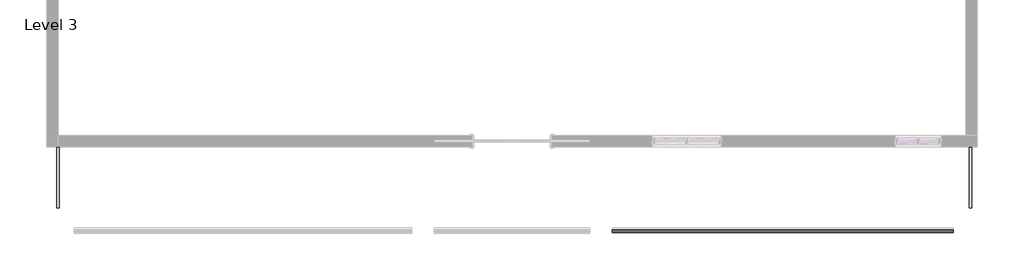
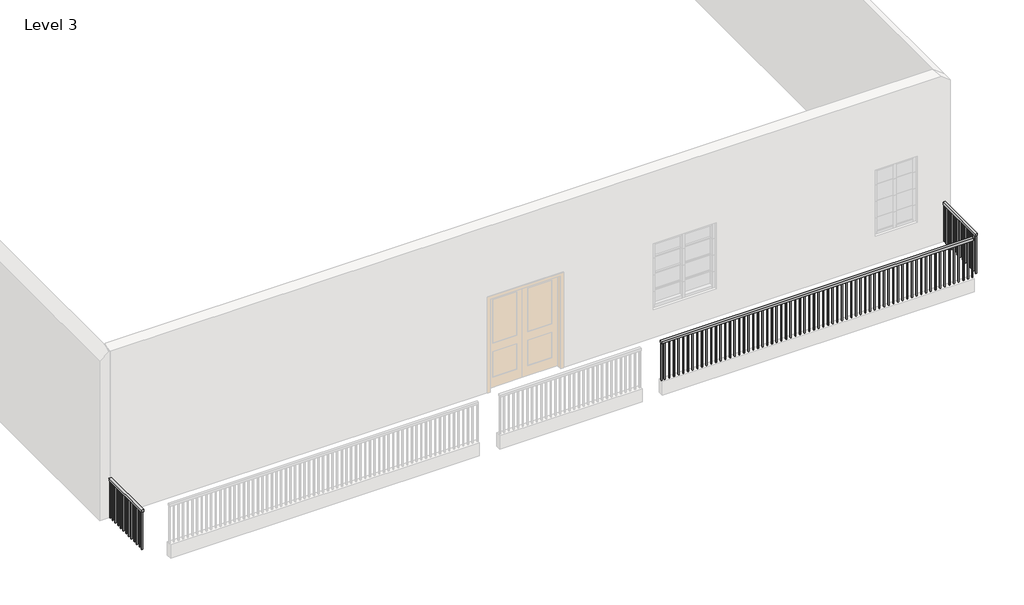
# One storey, part 3 of 3: 3 railings.
"""IFC4 building model written with IfcOpenShell, lengths in millimetres."""

from ifc_helpers import new_model, si_unit, frame, origin, place, context, project, spatial, polyline, outline, extrude, element, save

model = new_model("IFC4")

# Units and contexts
model_context = context("Model", 3, world=origin())
ifc_project = project(units=[si_unit("LENGTHUNIT", "METRE", prefix="MILLI")], contexts=[model_context])

# Site, building, storey
site = spatial("IfcSite", under=ifc_project)
building = spatial("IfcBuilding", under=site)
storey = spatial("IfcBuildingStorey", under=building, Name="Level 3", Elevation=3810.0)

# Railings
placement = place(None, origin())
element("IfcRailing", 1, ObjectType="Handrail - Rectangular", at=placement, inside=storey, context=model_context, shape_type="SweptSolid", body=[
    extrude(outline(polyline([(8263.5579341, -8749.7902135), (8263.5579341, -8800.5902135), (1481.7579341, -8800.5902135), (1481.7579341, -8749.7902135), (8263.5579341, -8749.7902135)])), frame((0.0, 0.0, 4978.4), z_axis=(0.0, 0.0, 1.0), x_axis=(1.0, 0.0, 0.0)), (0.0, 0.0, 1.0), 50.8),
    extrude(outline(polyline([(1567.4829341, -8765.6652135), (1567.4829341, -8784.7152135), (1548.4329341, -8784.7152135), (1548.4329341, -8765.6652135), (1567.4829341, -8765.6652135)])), frame((0.0, 0.0, 4114.8), z_axis=(0.0, 0.0, 1.0), x_axis=(1.0, 0.0, 0.0)), (0.0, 0.0, 1.0), 863.6),
    extrude(outline(polyline([(1669.0829341, -8765.6652135), (1669.0829341, -8784.7152135), (1650.0329341, -8784.7152135), (1650.0329341, -8765.6652135), (1669.0829341, -8765.6652135)])), frame((0.0, 0.0, 4114.8), z_axis=(0.0, 0.0, 1.0), x_axis=(1.0, 0.0, 0.0)), (0.0, 0.0, 1.0), 863.6),
    extrude(outline(polyline([(1770.6829341, -8765.6652135), (1770.6829341, -8784.7152135), (1751.6329341, -8784.7152135), (1751.6329341, -8765.6652135), (1770.6829341, -8765.6652135)])), frame((0.0, 0.0, 4114.8), z_axis=(0.0, 0.0, 1.0), x_axis=(1.0, 0.0, 0.0)), (0.0, 0.0, 1.0), 863.6),
    extrude(outline(polyline([(1872.2829341, -8765.6652135), (1872.2829341, -8784.7152135), (1853.2329341, -8784.7152135), (1853.2329341, -8765.6652135), (1872.2829341, -8765.6652135)])), frame((0.0, 0.0, 4114.8), z_axis=(0.0, 0.0, 1.0), x_axis=(1.0, 0.0, 0.0)), (0.0, 0.0, 1.0), 863.6),
    extrude(outline(polyline([(1973.8829341, -8765.6652135), (1973.8829341, -8784.7152135), (1954.8329341, -8784.7152135), (1954.8329341, -8765.6652135), (1973.8829341, -8765.6652135)])), frame((0.0, 0.0, 4114.8), z_axis=(0.0, 0.0, 1.0), x_axis=(1.0, 0.0, 0.0)), (0.0, 0.0, 1.0), 863.6),
    extrude(outline(polyline([(2075.4829341, -8765.6652135), (2075.4829341, -8784.7152135), (2056.4329341, -8784.7152135), (2056.4329341, -8765.6652135), (2075.4829341, -8765.6652135)])), frame((0.0, 0.0, 4114.8), z_axis=(0.0, 0.0, 1.0), x_axis=(1.0, 0.0, 0.0)), (0.0, 0.0, 1.0), 863.6),
    extrude(outline(polyline([(2177.0829341, -8765.6652135), (2177.0829341, -8784.7152135), (2158.0329341, -8784.7152135), (2158.0329341, -8765.6652135), (2177.0829341, -8765.6652135)])), frame((0.0, 0.0, 4114.8), z_axis=(0.0, 0.0, 1.0), x_axis=(1.0, 0.0, 0.0)), (0.0, 0.0, 1.0), 863.6),
    extrude(outline(polyline([(2278.6829341, -8765.6652135), (2278.6829341, -8784.7152135), (2259.6329341, -8784.7152135), (2259.6329341, -8765.6652135), (2278.6829341, -8765.6652135)])), frame((0.0, 0.0, 4114.8), z_axis=(0.0, 0.0, 1.0), x_axis=(1.0, 0.0, 0.0)), (0.0, 0.0, 1.0), 863.6),
    extrude(outline(polyline([(2380.2829341, -8765.6652135), (2380.2829341, -8784.7152135), (2361.2329341, -8784.7152135), (2361.2329341, -8765.6652135), (2380.2829341, -8765.6652135)])), frame((0.0, 0.0, 4114.8), z_axis=(0.0, 0.0, 1.0), x_axis=(1.0, 0.0, 0.0)), (0.0, 0.0, 1.0), 863.6),
    extrude(outline(polyline([(2481.8829341, -8765.6652135), (2481.8829341, -8784.7152135), (2462.8329341, -8784.7152135), (2462.8329341, -8765.6652135), (2481.8829341, -8765.6652135)])), frame((0.0, 0.0, 4114.8), z_axis=(0.0, 0.0, 1.0), x_axis=(1.0, 0.0, 0.0)), (0.0, 0.0, 1.0), 863.6),
    extrude(outline(polyline([(2583.4829341, -8765.6652135), (2583.4829341, -8784.7152135), (2564.4329341, -8784.7152135), (2564.4329341, -8765.6652135), (2583.4829341, -8765.6652135)])), frame((0.0, 0.0, 4114.8), z_axis=(0.0, 0.0, 1.0), x_axis=(1.0, 0.0, 0.0)), (0.0, 0.0, 1.0), 863.6),
    extrude(outline(polyline([(2685.0829341, -8765.6652135), (2685.0829341, -8784.7152135), (2666.0329341, -8784.7152135), (2666.0329341, -8765.6652135), (2685.0829341, -8765.6652135)])), frame((0.0, 0.0, 4114.8), z_axis=(0.0, 0.0, 1.0), x_axis=(1.0, 0.0, 0.0)), (0.0, 0.0, 1.0), 863.6),
    extrude(outline(polyline([(2786.6829341, -8765.6652135), (2786.6829341, -8784.7152135), (2767.6329341, -8784.7152135), (2767.6329341, -8765.6652135), (2786.6829341, -8765.6652135)])), frame((0.0, 0.0, 4114.8), z_axis=(0.0, 0.0, 1.0), x_axis=(1.0, 0.0, 0.0)), (0.0, 0.0, 1.0), 863.6),
    extrude(outline(polyline([(2888.2829341, -8765.6652135), (2888.2829341, -8784.7152135), (2869.2329341, -8784.7152135), (2869.2329341, -8765.6652135), (2888.2829341, -8765.6652135)])), frame((0.0, 0.0, 4114.8), z_axis=(0.0, 0.0, 1.0), x_axis=(1.0, 0.0, 0.0)), (0.0, 0.0, 1.0), 863.6),
    extrude(outline(polyline([(2989.8829341, -8765.6652135), (2989.8829341, -8784.7152135), (2970.8329341, -8784.7152135), (2970.8329341, -8765.6652135), (2989.8829341, -8765.6652135)])), frame((0.0, 0.0, 4114.8), z_axis=(0.0, 0.0, 1.0), x_axis=(1.0, 0.0, 0.0)), (0.0, 0.0, 1.0), 863.6),
    extrude(outline(polyline([(3091.4829341, -8765.6652135), (3091.4829341, -8784.7152135), (3072.4329341, -8784.7152135), (3072.4329341, -8765.6652135), (3091.4829341, -8765.6652135)])), frame((0.0, 0.0, 4114.8), z_axis=(0.0, 0.0, 1.0), x_axis=(1.0, 0.0, 0.0)), (0.0, 0.0, 1.0), 863.6),
    extrude(outline(polyline([(3193.0829341, -8765.6652135), (3193.0829341, -8784.7152135), (3174.0329341, -8784.7152135), (3174.0329341, -8765.6652135), (3193.0829341, -8765.6652135)])), frame((0.0, 0.0, 4114.8), z_axis=(0.0, 0.0, 1.0), x_axis=(1.0, 0.0, 0.0)), (0.0, 0.0, 1.0), 863.6),
    extrude(outline(polyline([(3294.6829341, -8765.6652135), (3294.6829341, -8784.7152135), (3275.6329341, -8784.7152135), (3275.6329341, -8765.6652135), (3294.6829341, -8765.6652135)])), frame((0.0, 0.0, 4114.8), z_axis=(0.0, 0.0, 1.0), x_axis=(1.0, 0.0, 0.0)), (0.0, 0.0, 1.0), 863.6),
    extrude(outline(polyline([(3396.2829341, -8765.6652135), (3396.2829341, -8784.7152135), (3377.2329341, -8784.7152135), (3377.2329341, -8765.6652135), (3396.2829341, -8765.6652135)])), frame((0.0, 0.0, 4114.8), z_axis=(0.0, 0.0, 1.0), x_axis=(1.0, 0.0, 0.0)), (0.0, 0.0, 1.0), 863.6),
    extrude(outline(polyline([(3497.8829341, -8765.6652135), (3497.8829341, -8784.7152135), (3478.8329341, -8784.7152135), (3478.8329341, -8765.6652135), (3497.8829341, -8765.6652135)])), frame((0.0, 0.0, 4114.8), z_axis=(0.0, 0.0, 1.0), x_axis=(1.0, 0.0, 0.0)), (0.0, 0.0, 1.0), 863.6),
    extrude(outline(polyline([(3599.4829341, -8765.6652135), (3599.4829341, -8784.7152135), (3580.4329341, -8784.7152135), (3580.4329341, -8765.6652135), (3599.4829341, -8765.6652135)])), frame((0.0, 0.0, 4114.8), z_axis=(0.0, 0.0, 1.0), x_axis=(1.0, 0.0, 0.0)), (0.0, 0.0, 1.0), 863.6),
    extrude(outline(polyline([(3701.0829341, -8765.6652135), (3701.0829341, -8784.7152135), (3682.0329341, -8784.7152135), (3682.0329341, -8765.6652135), (3701.0829341, -8765.6652135)])), frame((0.0, 0.0, 4114.8), z_axis=(0.0, 0.0, 1.0), x_axis=(1.0, 0.0, 0.0)), (0.0, 0.0, 1.0), 863.6),
    extrude(outline(polyline([(3802.6829341, -8765.6652135), (3802.6829341, -8784.7152135), (3783.6329341, -8784.7152135), (3783.6329341, -8765.6652135), (3802.6829341, -8765.6652135)])), frame((0.0, 0.0, 4114.8), z_axis=(0.0, 0.0, 1.0), x_axis=(1.0, 0.0, 0.0)), (0.0, 0.0, 1.0), 863.6),
    extrude(outline(polyline([(3904.2829341, -8765.6652135), (3904.2829341, -8784.7152135), (3885.2329341, -8784.7152135), (3885.2329341, -8765.6652135), (3904.2829341, -8765.6652135)])), frame((0.0, 0.0, 4114.8), z_axis=(0.0, 0.0, 1.0), x_axis=(1.0, 0.0, 0.0)), (0.0, 0.0, 1.0), 863.6),
    extrude(outline(polyline([(4005.8829341, -8765.6652135), (4005.8829341, -8784.7152135), (3986.8329341, -8784.7152135), (3986.8329341, -8765.6652135), (4005.8829341, -8765.6652135)])), frame((0.0, 0.0, 4114.8), z_axis=(0.0, 0.0, 1.0), x_axis=(1.0, 0.0, 0.0)), (0.0, 0.0, 1.0), 863.6),
    extrude(outline(polyline([(4107.4829341, -8765.6652135), (4107.4829341, -8784.7152135), (4088.4329341, -8784.7152135), (4088.4329341, -8765.6652135), (4107.4829341, -8765.6652135)])), frame((0.0, 0.0, 4114.8), z_axis=(0.0, 0.0, 1.0), x_axis=(1.0, 0.0, 0.0)), (0.0, 0.0, 1.0), 863.6),
    extrude(outline(polyline([(4209.0829341, -8765.6652135), (4209.0829341, -8784.7152135), (4190.0329341, -8784.7152135), (4190.0329341, -8765.6652135), (4209.0829341, -8765.6652135)])), frame((0.0, 0.0, 4114.8), z_axis=(0.0, 0.0, 1.0), x_axis=(1.0, 0.0, 0.0)), (0.0, 0.0, 1.0), 863.6),
    extrude(outline(polyline([(4310.6829341, -8765.6652135), (4310.6829341, -8784.7152135), (4291.6329341, -8784.7152135), (4291.6329341, -8765.6652135), (4310.6829341, -8765.6652135)])), frame((0.0, 0.0, 4114.8), z_axis=(0.0, 0.0, 1.0), x_axis=(1.0, 0.0, 0.0)), (0.0, 0.0, 1.0), 863.6),
    extrude(outline(polyline([(4412.2829341, -8765.6652135), (4412.2829341, -8784.7152135), (4393.2329341, -8784.7152135), (4393.2329341, -8765.6652135), (4412.2829341, -8765.6652135)])), frame((0.0, 0.0, 4114.8), z_axis=(0.0, 0.0, 1.0), x_axis=(1.0, 0.0, 0.0)), (0.0, 0.0, 1.0), 863.6),
    extrude(outline(polyline([(4513.8829341, -8765.6652135), (4513.8829341, -8784.7152135), (4494.8329341, -8784.7152135), (4494.8329341, -8765.6652135), (4513.8829341, -8765.6652135)])), frame((0.0, 0.0, 4114.8), z_axis=(0.0, 0.0, 1.0), x_axis=(1.0, 0.0, 0.0)), (0.0, 0.0, 1.0), 863.6),
    extrude(outline(polyline([(4615.4829341, -8765.6652135), (4615.4829341, -8784.7152135), (4596.4329341, -8784.7152135), (4596.4329341, -8765.6652135), (4615.4829341, -8765.6652135)])), frame((0.0, 0.0, 4114.8), z_axis=(0.0, 0.0, 1.0), x_axis=(1.0, 0.0, 0.0)), (0.0, 0.0, 1.0), 863.6),
    extrude(outline(polyline([(4717.0829341, -8765.6652135), (4717.0829341, -8784.7152135), (4698.0329341, -8784.7152135), (4698.0329341, -8765.6652135), (4717.0829341, -8765.6652135)])), frame((0.0, 0.0, 4114.8), z_axis=(0.0, 0.0, 1.0), x_axis=(1.0, 0.0, 0.0)), (0.0, 0.0, 1.0), 863.6),
    extrude(outline(polyline([(4818.6829341, -8765.6652135), (4818.6829341, -8784.7152135), (4799.6329341, -8784.7152135), (4799.6329341, -8765.6652135), (4818.6829341, -8765.6652135)])), frame((0.0, 0.0, 4114.8), z_axis=(0.0, 0.0, 1.0), x_axis=(1.0, 0.0, 0.0)), (0.0, 0.0, 1.0), 863.6),
    extrude(outline(polyline([(4920.2829341, -8765.6652135), (4920.2829341, -8784.7152135), (4901.2329341, -8784.7152135), (4901.2329341, -8765.6652135), (4920.2829341, -8765.6652135)])), frame((0.0, 0.0, 4114.8), z_axis=(0.0, 0.0, 1.0), x_axis=(1.0, 0.0, 0.0)), (0.0, 0.0, 1.0), 863.6),
    extrude(outline(polyline([(5021.8829341, -8765.6652135), (5021.8829341, -8784.7152135), (5002.8329341, -8784.7152135), (5002.8329341, -8765.6652135), (5021.8829341, -8765.6652135)])), frame((0.0, 0.0, 4114.8), z_axis=(0.0, 0.0, 1.0), x_axis=(1.0, 0.0, 0.0)), (0.0, 0.0, 1.0), 863.6),
    extrude(outline(polyline([(5123.4829341, -8765.6652135), (5123.4829341, -8784.7152135), (5104.4329341, -8784.7152135), (5104.4329341, -8765.6652135), (5123.4829341, -8765.6652135)])), frame((0.0, 0.0, 4114.8), z_axis=(0.0, 0.0, 1.0), x_axis=(1.0, 0.0, 0.0)), (0.0, 0.0, 1.0), 863.6),
    extrude(outline(polyline([(5225.0829341, -8765.6652135), (5225.0829341, -8784.7152135), (5206.0329341, -8784.7152135), (5206.0329341, -8765.6652135), (5225.0829341, -8765.6652135)])), frame((0.0, 0.0, 4114.8), z_axis=(0.0, 0.0, 1.0), x_axis=(1.0, 0.0, 0.0)), (0.0, 0.0, 1.0), 863.6),
    extrude(outline(polyline([(5326.6829341, -8765.6652135), (5326.6829341, -8784.7152135), (5307.6329341, -8784.7152135), (5307.6329341, -8765.6652135), (5326.6829341, -8765.6652135)])), frame((0.0, 0.0, 4114.8), z_axis=(0.0, 0.0, 1.0), x_axis=(1.0, 0.0, 0.0)), (0.0, 0.0, 1.0), 863.6),
    extrude(outline(polyline([(5428.2829341, -8765.6652135), (5428.2829341, -8784.7152135), (5409.2329341, -8784.7152135), (5409.2329341, -8765.6652135), (5428.2829341, -8765.6652135)])), frame((0.0, 0.0, 4114.8), z_axis=(0.0, 0.0, 1.0), x_axis=(1.0, 0.0, 0.0)), (0.0, 0.0, 1.0), 863.6),
    extrude(outline(polyline([(5529.8829341, -8765.6652135), (5529.8829341, -8784.7152135), (5510.8329341, -8784.7152135), (5510.8329341, -8765.6652135), (5529.8829341, -8765.6652135)])), frame((0.0, 0.0, 4114.8), z_axis=(0.0, 0.0, 1.0), x_axis=(1.0, 0.0, 0.0)), (0.0, 0.0, 1.0), 863.6),
    extrude(outline(polyline([(5631.4829341, -8765.6652135), (5631.4829341, -8784.7152135), (5612.4329341, -8784.7152135), (5612.4329341, -8765.6652135), (5631.4829341, -8765.6652135)])), frame((0.0, 0.0, 4114.8), z_axis=(0.0, 0.0, 1.0), x_axis=(1.0, 0.0, 0.0)), (0.0, 0.0, 1.0), 863.6),
    extrude(outline(polyline([(5733.0829341, -8765.6652135), (5733.0829341, -8784.7152135), (5714.0329341, -8784.7152135), (5714.0329341, -8765.6652135), (5733.0829341, -8765.6652135)])), frame((0.0, 0.0, 4114.8), z_axis=(0.0, 0.0, 1.0), x_axis=(1.0, 0.0, 0.0)), (0.0, 0.0, 1.0), 863.6),
    extrude(outline(polyline([(5834.6829341, -8765.6652135), (5834.6829341, -8784.7152135), (5815.6329341, -8784.7152135), (5815.6329341, -8765.6652135), (5834.6829341, -8765.6652135)])), frame((0.0, 0.0, 4114.8), z_axis=(0.0, 0.0, 1.0), x_axis=(1.0, 0.0, 0.0)), (0.0, 0.0, 1.0), 863.6),
    extrude(outline(polyline([(5936.2829341, -8765.6652135), (5936.2829341, -8784.7152135), (5917.2329341, -8784.7152135), (5917.2329341, -8765.6652135), (5936.2829341, -8765.6652135)])), frame((0.0, 0.0, 4114.8), z_axis=(0.0, 0.0, 1.0), x_axis=(1.0, 0.0, 0.0)), (0.0, 0.0, 1.0), 863.6),
    extrude(outline(polyline([(6037.8829341, -8765.6652135), (6037.8829341, -8784.7152135), (6018.8329341, -8784.7152135), (6018.8329341, -8765.6652135), (6037.8829341, -8765.6652135)])), frame((0.0, 0.0, 4114.8), z_axis=(0.0, 0.0, 1.0), x_axis=(1.0, 0.0, 0.0)), (0.0, 0.0, 1.0), 863.6),
    extrude(outline(polyline([(6139.4829341, -8765.6652135), (6139.4829341, -8784.7152135), (6120.4329341, -8784.7152135), (6120.4329341, -8765.6652135), (6139.4829341, -8765.6652135)])), frame((0.0, 0.0, 4114.8), z_axis=(0.0, 0.0, 1.0), x_axis=(1.0, 0.0, 0.0)), (0.0, 0.0, 1.0), 863.6),
    extrude(outline(polyline([(6241.0829341, -8765.6652135), (6241.0829341, -8784.7152135), (6222.0329341, -8784.7152135), (6222.0329341, -8765.6652135), (6241.0829341, -8765.6652135)])), frame((0.0, 0.0, 4114.8), z_axis=(0.0, 0.0, 1.0), x_axis=(1.0, 0.0, 0.0)), (0.0, 0.0, 1.0), 863.6),
    extrude(outline(polyline([(6342.6829341, -8765.6652135), (6342.6829341, -8784.7152135), (6323.6329341, -8784.7152135), (6323.6329341, -8765.6652135), (6342.6829341, -8765.6652135)])), frame((0.0, 0.0, 4114.8), z_axis=(0.0, 0.0, 1.0), x_axis=(1.0, 0.0, 0.0)), (0.0, 0.0, 1.0), 863.6),
    extrude(outline(polyline([(6444.2829341, -8765.6652135), (6444.2829341, -8784.7152135), (6425.2329341, -8784.7152135), (6425.2329341, -8765.6652135), (6444.2829341, -8765.6652135)])), frame((0.0, 0.0, 4114.8), z_axis=(0.0, 0.0, 1.0), x_axis=(1.0, 0.0, 0.0)), (0.0, 0.0, 1.0), 863.6),
    extrude(outline(polyline([(6545.8829341, -8765.6652135), (6545.8829341, -8784.7152135), (6526.8329341, -8784.7152135), (6526.8329341, -8765.6652135), (6545.8829341, -8765.6652135)])), frame((0.0, 0.0, 4114.8), z_axis=(0.0, 0.0, 1.0), x_axis=(1.0, 0.0, 0.0)), (0.0, 0.0, 1.0), 863.6),
    extrude(outline(polyline([(6647.4829341, -8765.6652135), (6647.4829341, -8784.7152135), (6628.4329341, -8784.7152135), (6628.4329341, -8765.6652135), (6647.4829341, -8765.6652135)])), frame((0.0, 0.0, 4114.8), z_axis=(0.0, 0.0, 1.0), x_axis=(1.0, 0.0, 0.0)), (0.0, 0.0, 1.0), 863.6),
    extrude(outline(polyline([(6749.0829341, -8765.6652135), (6749.0829341, -8784.7152135), (6730.0329341, -8784.7152135), (6730.0329341, -8765.6652135), (6749.0829341, -8765.6652135)])), frame((0.0, 0.0, 4114.8), z_axis=(0.0, 0.0, 1.0), x_axis=(1.0, 0.0, 0.0)), (0.0, 0.0, 1.0), 863.6),
    extrude(outline(polyline([(6850.6829341, -8765.6652135), (6850.6829341, -8784.7152135), (6831.6329341, -8784.7152135), (6831.6329341, -8765.6652135), (6850.6829341, -8765.6652135)])), frame((0.0, 0.0, 4114.8), z_axis=(0.0, 0.0, 1.0), x_axis=(1.0, 0.0, 0.0)), (0.0, 0.0, 1.0), 863.6),
    extrude(outline(polyline([(6952.2829341, -8765.6652135), (6952.2829341, -8784.7152135), (6933.2329341, -8784.7152135), (6933.2329341, -8765.6652135), (6952.2829341, -8765.6652135)])), frame((0.0, 0.0, 4114.8), z_axis=(0.0, 0.0, 1.0), x_axis=(1.0, 0.0, 0.0)), (0.0, 0.0, 1.0), 863.6),
    extrude(outline(polyline([(7053.8829341, -8765.6652135), (7053.8829341, -8784.7152135), (7034.8329341, -8784.7152135), (7034.8329341, -8765.6652135), (7053.8829341, -8765.6652135)])), frame((0.0, 0.0, 4114.8), z_axis=(0.0, 0.0, 1.0), x_axis=(1.0, 0.0, 0.0)), (0.0, 0.0, 1.0), 863.6),
    extrude(outline(polyline([(7155.4829341, -8765.6652135), (7155.4829341, -8784.7152135), (7136.4329341, -8784.7152135), (7136.4329341, -8765.6652135), (7155.4829341, -8765.6652135)])), frame((0.0, 0.0, 4114.8), z_axis=(0.0, 0.0, 1.0), x_axis=(1.0, 0.0, 0.0)), (0.0, 0.0, 1.0), 863.6),
    extrude(outline(polyline([(7257.0829341, -8765.6652135), (7257.0829341, -8784.7152135), (7238.0329341, -8784.7152135), (7238.0329341, -8765.6652135), (7257.0829341, -8765.6652135)])), frame((0.0, 0.0, 4114.8), z_axis=(0.0, 0.0, 1.0), x_axis=(1.0, 0.0, 0.0)), (0.0, 0.0, 1.0), 863.6),
    extrude(outline(polyline([(7358.6829341, -8765.6652135), (7358.6829341, -8784.7152135), (7339.6329341, -8784.7152135), (7339.6329341, -8765.6652135), (7358.6829341, -8765.6652135)])), frame((0.0, 0.0, 4114.8), z_axis=(0.0, 0.0, 1.0), x_axis=(1.0, 0.0, 0.0)), (0.0, 0.0, 1.0), 863.6),
    extrude(outline(polyline([(7460.2829341, -8765.6652135), (7460.2829341, -8784.7152135), (7441.2329341, -8784.7152135), (7441.2329341, -8765.6652135), (7460.2829341, -8765.6652135)])), frame((0.0, 0.0, 4114.8), z_axis=(0.0, 0.0, 1.0), x_axis=(1.0, 0.0, 0.0)), (0.0, 0.0, 1.0), 863.6),
    extrude(outline(polyline([(7561.8829341, -8765.6652135), (7561.8829341, -8784.7152135), (7542.8329341, -8784.7152135), (7542.8329341, -8765.6652135), (7561.8829341, -8765.6652135)])), frame((0.0, 0.0, 4114.8), z_axis=(0.0, 0.0, 1.0), x_axis=(1.0, 0.0, 0.0)), (0.0, 0.0, 1.0), 863.6),
    extrude(outline(polyline([(7663.4829341, -8765.6652135), (7663.4829341, -8784.7152135), (7644.4329341, -8784.7152135), (7644.4329341, -8765.6652135), (7663.4829341, -8765.6652135)])), frame((0.0, 0.0, 4114.8), z_axis=(0.0, 0.0, 1.0), x_axis=(1.0, 0.0, 0.0)), (0.0, 0.0, 1.0), 863.6),
    extrude(outline(polyline([(7765.0829341, -8765.6652135), (7765.0829341, -8784.7152135), (7746.0329341, -8784.7152135), (7746.0329341, -8765.6652135), (7765.0829341, -8765.6652135)])), frame((0.0, 0.0, 4114.8), z_axis=(0.0, 0.0, 1.0), x_axis=(1.0, 0.0, 0.0)), (0.0, 0.0, 1.0), 863.6),
    extrude(outline(polyline([(7866.6829341, -8765.6652135), (7866.6829341, -8784.7152135), (7847.6329341, -8784.7152135), (7847.6329341, -8765.6652135), (7866.6829341, -8765.6652135)])), frame((0.0, 0.0, 4114.8), z_axis=(0.0, 0.0, 1.0), x_axis=(1.0, 0.0, 0.0)), (0.0, 0.0, 1.0), 863.6),
    extrude(outline(polyline([(7968.2829341, -8765.6652135), (7968.2829341, -8784.7152135), (7949.2329341, -8784.7152135), (7949.2329341, -8765.6652135), (7968.2829341, -8765.6652135)])), frame((0.0, 0.0, 4114.8), z_axis=(0.0, 0.0, 1.0), x_axis=(1.0, 0.0, 0.0)), (0.0, 0.0, 1.0), 863.6),
    extrude(outline(polyline([(8069.8829341, -8765.6652135), (8069.8829341, -8784.7152135), (8050.8329341, -8784.7152135), (8050.8329341, -8765.6652135), (8069.8829341, -8765.6652135)])), frame((0.0, 0.0, 4114.8), z_axis=(0.0, 0.0, 1.0), x_axis=(1.0, 0.0, 0.0)), (0.0, 0.0, 1.0), 863.6),
    extrude(outline(polyline([(8171.4829341, -8765.6652135), (8171.4829341, -8784.7152135), (8152.4329341, -8784.7152135), (8152.4329341, -8765.6652135), (8171.4829341, -8765.6652135)])), frame((0.0, 0.0, 4114.8), z_axis=(0.0, 0.0, 1.0), x_axis=(1.0, 0.0, 0.0)), (0.0, 0.0, 1.0), 863.6),
    extrude(outline(polyline([(1500.8079341, -8765.6652135), (1500.8079341, -8784.7152135), (1481.7579341, -8784.7152135), (1481.7579341, -8765.6652135), (1500.8079341, -8765.6652135)])), frame((0.0, 0.0, 4114.8), z_axis=(0.0, 0.0, 1.0), x_axis=(1.0, 0.0, 0.0)), (0.0, 0.0, 1.0), 863.6),
    extrude(outline(polyline([(8263.5579341, -8765.6652135), (8263.5579341, -8784.7152135), (8244.5079341, -8784.7152135), (8244.5079341, -8765.6652135), (8263.5579341, -8765.6652135)])), frame((0.0, 0.0, 4114.8), z_axis=(0.0, 0.0, 1.0), x_axis=(1.0, 0.0, 0.0)), (0.0, 0.0, 1.0), 863.6),
])
element("IfcRailing", 2, ObjectType="Handrail - Rectangular", at=placement, inside=storey, context=model_context, shape_type="SweptSolid", body=[
    extrude(outline(polyline([(8581.0579341, -7100.4878342), (8631.8579341, -7100.4878342), (8631.8579341, -8317.9902135), (8581.0579341, -8317.9902135), (8581.0579341, -7100.4878342)])), frame((0.0, 0.0, 4673.6), z_axis=(0.0, 0.0, 1.0), x_axis=(1.0, 0.0, 0.0)), (0.0, 0.0, 1.0), 50.8),
    extrude(outline(polyline([(8596.9329341, -8208.5628342), (8615.9829341, -8208.5628342), (8615.9829341, -8227.6128342), (8596.9329341, -8227.6128342), (8596.9329341, -8208.5628342)])), frame((0.0, 0.0, 3810.0), z_axis=(0.0, 0.0, 1.0), x_axis=(1.0, 0.0, 0.0)), (0.0, 0.0, 1.0), 863.6),
    extrude(outline(polyline([(8596.9329341, -8106.9628342), (8615.9829341, -8106.9628342), (8615.9829341, -8126.0128342), (8596.9329341, -8126.0128342), (8596.9329341, -8106.9628342)])), frame((0.0, 0.0, 3810.0), z_axis=(0.0, 0.0, 1.0), x_axis=(1.0, 0.0, 0.0)), (0.0, 0.0, 1.0), 863.6),
    extrude(outline(polyline([(8596.9329341, -8005.3628342), (8615.9829341, -8005.3628342), (8615.9829341, -8024.4128342), (8596.9329341, -8024.4128342), (8596.9329341, -8005.3628342)])), frame((0.0, 0.0, 3810.0), z_axis=(0.0, 0.0, 1.0), x_axis=(1.0, 0.0, 0.0)), (0.0, 0.0, 1.0), 863.6),
    extrude(outline(polyline([(8596.9329341, -7903.7628342), (8615.9829341, -7903.7628342), (8615.9829341, -7922.8128342), (8596.9329341, -7922.8128342), (8596.9329341, -7903.7628342)])), frame((0.0, 0.0, 3810.0), z_axis=(0.0, 0.0, 1.0), x_axis=(1.0, 0.0, 0.0)), (0.0, 0.0, 1.0), 863.6),
    extrude(outline(polyline([(8596.9329341, -7802.1628342), (8615.9829341, -7802.1628342), (8615.9829341, -7821.2128342), (8596.9329341, -7821.2128342), (8596.9329341, -7802.1628342)])), frame((0.0, 0.0, 3810.0), z_axis=(0.0, 0.0, 1.0), x_axis=(1.0, 0.0, 0.0)), (0.0, 0.0, 1.0), 863.6),
    extrude(outline(polyline([(8596.9329341, -7700.5628342), (8615.9829341, -7700.5628342), (8615.9829341, -7719.6128342), (8596.9329341, -7719.6128342), (8596.9329341, -7700.5628342)])), frame((0.0, 0.0, 3810.0), z_axis=(0.0, 0.0, 1.0), x_axis=(1.0, 0.0, 0.0)), (0.0, 0.0, 1.0), 863.6),
    extrude(outline(polyline([(8596.9329341, -7598.9628342), (8615.9829341, -7598.9628342), (8615.9829341, -7618.0128342), (8596.9329341, -7618.0128342), (8596.9329341, -7598.9628342)])), frame((0.0, 0.0, 3810.0), z_axis=(0.0, 0.0, 1.0), x_axis=(1.0, 0.0, 0.0)), (0.0, 0.0, 1.0), 863.6),
    extrude(outline(polyline([(8596.9329341, -7497.3628342), (8615.9829341, -7497.3628342), (8615.9829341, -7516.4128342), (8596.9329341, -7516.4128342), (8596.9329341, -7497.3628342)])), frame((0.0, 0.0, 3810.0), z_axis=(0.0, 0.0, 1.0), x_axis=(1.0, 0.0, 0.0)), (0.0, 0.0, 1.0), 863.6),
    extrude(outline(polyline([(8596.9329341, -7395.7628342), (8615.9829341, -7395.7628342), (8615.9829341, -7414.8128342), (8596.9329341, -7414.8128342), (8596.9329341, -7395.7628342)])), frame((0.0, 0.0, 3810.0), z_axis=(0.0, 0.0, 1.0), x_axis=(1.0, 0.0, 0.0)), (0.0, 0.0, 1.0), 863.6),
    extrude(outline(polyline([(8596.9329341, -7294.1628342), (8615.9829341, -7294.1628342), (8615.9829341, -7313.2128342), (8596.9329341, -7313.2128342), (8596.9329341, -7294.1628342)])), frame((0.0, 0.0, 3810.0), z_axis=(0.0, 0.0, 1.0), x_axis=(1.0, 0.0, 0.0)), (0.0, 0.0, 1.0), 863.6),
    extrude(outline(polyline([(8596.9329341, -7192.5628342), (8615.9829341, -7192.5628342), (8615.9829341, -7211.6128342), (8596.9329341, -7211.6128342), (8596.9329341, -7192.5628342)])), frame((0.0, 0.0, 3810.0), z_axis=(0.0, 0.0, 1.0), x_axis=(1.0, 0.0, 0.0)), (0.0, 0.0, 1.0), 863.6),
    extrude(outline(polyline([(8596.9329341, -8298.9402135), (8615.9829341, -8298.9402135), (8615.9829341, -8317.9902135), (8596.9329341, -8317.9902135), (8596.9329341, -8298.9402135)])), frame((0.0, 0.0, 3810.0), z_axis=(0.0, 0.0, 1.0), x_axis=(1.0, 0.0, 0.0)), (0.0, 0.0, 1.0), 863.6),
    extrude(outline(polyline([(8596.9329341, -7100.4878342), (8615.9829341, -7100.4878342), (8615.9829341, -7119.5378342), (8596.9329341, -7119.5378342), (8596.9329341, -7100.4878342)])), frame((0.0, 0.0, 3810.0), z_axis=(0.0, 0.0, 1.0), x_axis=(1.0, 0.0, 0.0)), (0.0, 0.0, 1.0), 863.6),
])
element("IfcRailing", 3, ObjectType="Handrail - Rectangular", at=placement, inside=storey, context=model_context, shape_type="SweptSolid", body=[
    extrude(outline(polyline([(-9567.2420659, -7100.4878342), (-9516.4420659, -7100.4878342), (-9516.4420659, -8317.9902135), (-9567.2420659, -8317.9902135), (-9567.2420659, -7100.4878342)])), frame((0.0, 0.0, 4673.6), z_axis=(0.0, 0.0, 1.0), x_axis=(1.0, 0.0, 0.0)), (0.0, 0.0, 1.0), 50.8),
    extrude(outline(polyline([(-9551.3670659, -8208.5628342), (-9532.3170659, -8208.5628342), (-9532.3170659, -8227.6128342), (-9551.3670659, -8227.6128342), (-9551.3670659, -8208.5628342)])), frame((0.0, 0.0, 3810.0), z_axis=(0.0, 0.0, 1.0), x_axis=(1.0, 0.0, 0.0)), (0.0, 0.0, 1.0), 863.6),
    extrude(outline(polyline([(-9551.3670659, -8106.9628342), (-9532.3170659, -8106.9628342), (-9532.3170659, -8126.0128342), (-9551.3670659, -8126.0128342), (-9551.3670659, -8106.9628342)])), frame((0.0, 0.0, 3810.0), z_axis=(0.0, 0.0, 1.0), x_axis=(1.0, 0.0, 0.0)), (0.0, 0.0, 1.0), 863.6),
    extrude(outline(polyline([(-9551.3670659, -8005.3628342), (-9532.3170659, -8005.3628342), (-9532.3170659, -8024.4128342), (-9551.3670659, -8024.4128342), (-9551.3670659, -8005.3628342)])), frame((0.0, 0.0, 3810.0), z_axis=(0.0, 0.0, 1.0), x_axis=(1.0, 0.0, 0.0)), (0.0, 0.0, 1.0), 863.6),
    extrude(outline(polyline([(-9551.3670659, -7903.7628342), (-9532.3170659, -7903.7628342), (-9532.3170659, -7922.8128342), (-9551.3670659, -7922.8128342), (-9551.3670659, -7903.7628342)])), frame((0.0, 0.0, 3810.0), z_axis=(0.0, 0.0, 1.0), x_axis=(1.0, 0.0, 0.0)), (0.0, 0.0, 1.0), 863.6),
    extrude(outline(polyline([(-9551.3670659, -7802.1628342), (-9532.3170659, -7802.1628342), (-9532.3170659, -7821.2128342), (-9551.3670659, -7821.2128342), (-9551.3670659, -7802.1628342)])), frame((0.0, 0.0, 3810.0), z_axis=(0.0, 0.0, 1.0), x_axis=(1.0, 0.0, 0.0)), (0.0, 0.0, 1.0), 863.6),
    extrude(outline(polyline([(-9551.3670659, -7700.5628342), (-9532.3170659, -7700.5628342), (-9532.3170659, -7719.6128342), (-9551.3670659, -7719.6128342), (-9551.3670659, -7700.5628342)])), frame((0.0, 0.0, 3810.0), z_axis=(0.0, 0.0, 1.0), x_axis=(1.0, 0.0, 0.0)), (0.0, 0.0, 1.0), 863.6),
    extrude(outline(polyline([(-9551.3670659, -7598.9628342), (-9532.3170659, -7598.9628342), (-9532.3170659, -7618.0128342), (-9551.3670659, -7618.0128342), (-9551.3670659, -7598.9628342)])), frame((0.0, 0.0, 3810.0), z_axis=(0.0, 0.0, 1.0), x_axis=(1.0, 0.0, 0.0)), (0.0, 0.0, 1.0), 863.6),
    extrude(outline(polyline([(-9551.3670659, -7497.3628342), (-9532.3170659, -7497.3628342), (-9532.3170659, -7516.4128342), (-9551.3670659, -7516.4128342), (-9551.3670659, -7497.3628342)])), frame((0.0, 0.0, 3810.0), z_axis=(0.0, 0.0, 1.0), x_axis=(1.0, 0.0, 0.0)), (0.0, 0.0, 1.0), 863.6),
    extrude(outline(polyline([(-9551.3670659, -7395.7628342), (-9532.3170659, -7395.7628342), (-9532.3170659, -7414.8128342), (-9551.3670659, -7414.8128342), (-9551.3670659, -7395.7628342)])), frame((0.0, 0.0, 3810.0), z_axis=(0.0, 0.0, 1.0), x_axis=(1.0, 0.0, 0.0)), (0.0, 0.0, 1.0), 863.6),
    extrude(outline(polyline([(-9551.3670659, -7294.1628342), (-9532.3170659, -7294.1628342), (-9532.3170659, -7313.2128342), (-9551.3670659, -7313.2128342), (-9551.3670659, -7294.1628342)])), frame((0.0, 0.0, 3810.0), z_axis=(0.0, 0.0, 1.0), x_axis=(1.0, 0.0, 0.0)), (0.0, 0.0, 1.0), 863.6),
    extrude(outline(polyline([(-9551.3670659, -7192.5628342), (-9532.3170659, -7192.5628342), (-9532.3170659, -7211.6128342), (-9551.3670659, -7211.6128342), (-9551.3670659, -7192.5628342)])), frame((0.0, 0.0, 3810.0), z_axis=(0.0, 0.0, 1.0), x_axis=(1.0, 0.0, 0.0)), (0.0, 0.0, 1.0), 863.6),
    extrude(outline(polyline([(-9551.3670659, -8298.9402135), (-9532.3170659, -8298.9402135), (-9532.3170659, -8317.9902135), (-9551.3670659, -8317.9902135), (-9551.3670659, -8298.9402135)])), frame((0.0, 0.0, 3810.0), z_axis=(0.0, 0.0, 1.0), x_axis=(1.0, 0.0, 0.0)), (0.0, 0.0, 1.0), 863.6),
    extrude(outline(polyline([(-9551.3670659, -7100.4878342), (-9532.3170659, -7100.4878342), (-9532.3170659, -7119.5378342), (-9551.3670659, -7119.5378342), (-9551.3670659, -7100.4878342)])), frame((0.0, 0.0, 3810.0), z_axis=(0.0, 0.0, 1.0), x_axis=(1.0, 0.0, 0.0)), (0.0, 0.0, 1.0), 863.6),
])

save(model, "model.ifc")

# Revit data of these elements
# Type "Handrail - Rectangular"
#   Assembly Code = "C2010400"
#   built-in parameter 1008612 = 0.0416667 (stored number, unit not read)
#   built-in parameter 1008611 = 0.0416667 (stored number, unit not read)
#   built-in parameter 1008609 = 0.333333 (stored number, unit not read)
#   built-in parameter 1008604 = 0.166667 (stored number, unit not read)
#   built-in parameter 1008603 = 0.166667 (stored number, unit not read)
#   Railing Height = 3' - 0"
#   built-in parameter 1008630 = 2
#   built-in parameter 1008610 = 2
#   built-in parameter 1008618 = Baluster - Square : 3/4"
# Element 1 (IfcRailing, "Handrail - Rectangular")
#   built-in parameter 1008621 = 1 (stored number, unit not read)
#   Phase Created = New Construction
# Elements 2, 3 (IfcRailing, "Handrail - Rectangular")
#   Phase Created = New Construction
